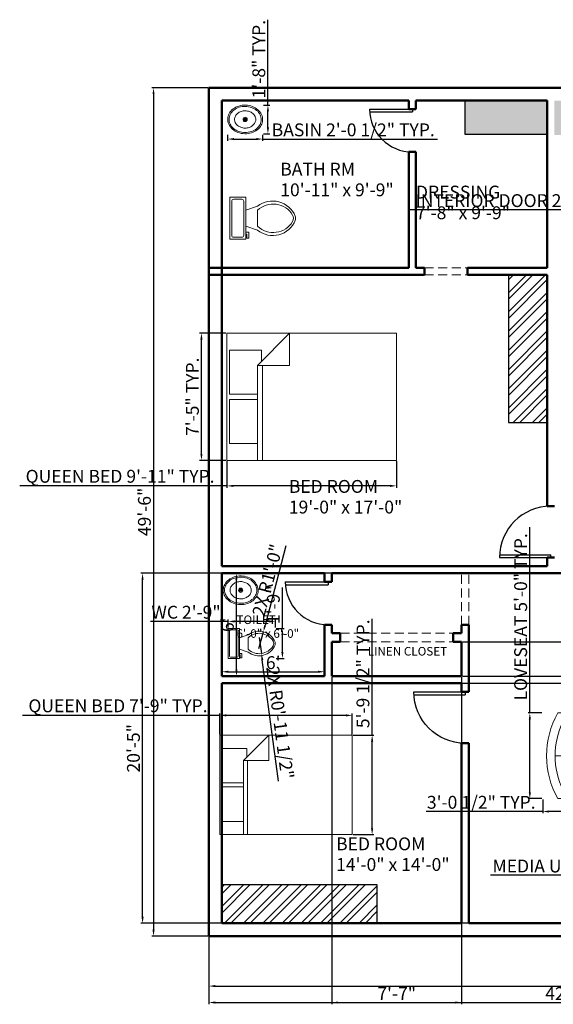
# Model space of a CAD drawing. Units: inches. Extents: x 2043 to 3102, y 1334 to 2053.
# Tile 1 of 4: x 2043 to 2416, y 1334 to 2024. Entities that reach past the tile are written whole.
import ezdxf

# ---------------------------------------------------------------- set-up
doc = ezdxf.new("R2010")
doc.units = ezdxf.units.IN
doc.linetypes.add('HIDDEN', pattern=[9.525, 6.35, -3.175])
for name, color, linetype, lineweight in [('A-ANNO-DIMS', 2, 'Continuous', 18), ('A-AREA-IDEN', 165, 'Continuous', 25), ('A-DOOR', 4, 'Continuous', 25), ('A-FLOR-CASE', 18, 'Continuous', 25), ('A-FLOR-CASE-PATT', 18, 'Continuous', 13), ('A-FLOR-FIXT', 9, 'Continuous', 20), ('A-FURN', 8, 'Continuous', 18), ('A-WALL', 7, 'Continuous', 50), ('A-WALL-OVHD', 11, 'HIDDEN', 18)]:
    doc.layers.add(name, color=color, linetype=linetype, lineweight=lineweight)
doc.styles.get("Standard").update_dxf_attribs({"font": 'arial.ttf'})
doc.dimstyles.new('ISO-25', dxfattribs={"dimtxt": 9, "dimasz": 4.5, "dimexe": 1.25, "dimexo": 0.625, "dimtad": 1, "dimdec": 0, "dimlunit": 3, "dimtxsty": 'Standard', "dimcen": 2.5, "dimadec": 0, "dimazin": 0, "dimtfac": 1, "dimtdec": 0, "dimtmove": 0, "dimatfit": 3, "dimfxl": 1, "dimarcsym": 0})

# ---------------------------------------------------------------- blocks, each defined once
blk = doc.blocks.new('Toilet - top')
for p, q in [((9.5, -6), (9.5, -2)), ((-10, -8.5), (-8, -8.5)), ((-10, -9.5), (-10, -8.5)), ((-7, -9.5), (-10, -9.5)), ((-8, -8.5), (-8, -8)), ((-7, -8), (-7, -9.5)), ((-4, -8), (-6, -14)), ((4, -8), (6, -14)), ((4, -14), (-4, -14))]:
    blk.add_line(p, q)
blk.add_lwpolyline([(10.5, -8), (10.5, 0), (-10.5, 0), (-10.5, -8)], close=True)
for points in [[(-9.5, -2), (-9.5, -6)], [(8.5, -1), (-8.5, -1)], [(-8.5, -7), (8.5, -7)]]:
    blk.add_lwpolyline(points)
for centre, radius, start, end in [((-8.62, -1.88), 0.884, 81.8699, 188.1301), ((8.62, -1.88), 0.884, 351.8699, 98.1301), ((-8.62, -6.12), 0.884, 171.8699, 278.1301), ((8.62, -6.12), 0.884, 261.8699, 8.1301), ((3.52, -21.58), 12.17, 141.4691, 247.9714), ((4.2, -21.82), 11.33, 136.3677, 238.9468), ((-3.52, -21.58), 12.17, 292.0284, 38.5307), ((-4.2, -21.82), 11.33, 301.053, 43.6321), ((0, -27.88), 4, 245.7318, 294.2682), ((0, -29), 4, 254.8605, 285.1395)]:
    blk.add_arc(centre, radius, start, end)
blk = doc.blocks.new('Bed - Queen')
for p, q in [((0, -80.00003), (0, 0)), ((0, 0), (59.99999, 0)), ((59.99999, 0), (59.99999, -80.00003)), ((7.99999, -1.2), (28.79998, -1.2)), ((7.99999, -14.4), (7.99999, -1.2)), ((28.79998, -1.2), (28.79998, -14.4)), ((31.19999, -1.2), (51.99999, -1.2)), ((31.19999, -14.4), (31.19999, -1.2)), ((51.99999, -1.2), (51.99999, -16.4)), ((0, -14.4), (44.8, -14.4)), ((44.8, -16.8), (0, -16.8)), ((59.99999, -29.6), (44.8, -14.4)), ((44.8, -14.4), (44.8, -29.6)), ((51.99999, -16.4), (46.79936, -16.4)), ((44.8, -29.6), (59.99999, -29.6)), ((59.99999, -80.00003), (0, -80.00003))]:
    blk.add_line(p, q)
blk = doc.blocks.new('Sofa - Roundback Loveseat 5 ft.')
for p, q in [((0, -32.44198), (0, -5.99998)), ((-24, -33.99998), (-24, -11.46958)), ((-23.9998, -13.38178), (23.99986, -13.38178)), ((24.00004, -33.99998), (24.00004, -11.46958)), ((-24, -32.44198), (24.00004, -32.44198))]:
    blk.add_line(p, q)
for points in [[(-24, -33.99998), (-30, -33.99998), (-30, -7.99998)], [(30.00004, -7.99998), (30.00004, -33.99998), (24.00004, -33.99998)]]:
    blk.add_lwpolyline(points)
for centre, radius, start, end in [((0, -60.24998), 60.24998, 60.13715, 119.8628), ((0, -61.38438), 55.38444, 64.32083, 115.6792)]:
    blk.add_arc(centre, radius, start, end)
blk = doc.blocks.new('Sink - Oval top')
for p, q in [((-1, 0), (1, 0)), ((0, 1), (0, -1))]:
    blk.add_line(p, q)
for points in [[(-12.23, 0.39, 0.117634), (-11.46, -3.36, 0.104469), (-8.88, -6.8, 0.090016), (-5.08, -9.07, 0.08192), (-0.32, -10.02, 0.08192), (4.49, -9.38, 0.090016), (8.42, -7.36, 0.104469), (11.22, -4.09, 0.117634), (12.23, -0.39, 0.117634), (11.46, 3.36, 0.104469), (8.88, 6.8, 0.090016), (5.08, 9.07, 0.08192), (0.32, 10.02, 0.08192), (-4.49, 9.38, 0.090016), (-8.42, 7.36, 0.104469), (-11.22, 4.09, 0.117634)], [(-11.29, 0.16, 0.118622), (-10.52, -3.25, 0.104678), (-8.07, -6.36, 0.089562), (-4.54, -8.37, 0.081185), (-0.13, -9.15, 0.081185), (4.3, -8.49, 0.089562), (7.89, -6.58, 0.104678), (10.42, -3.55, 0.118622), (11.29, -0.16, 0.118622), (10.52, 3.25, 0.104678), (8.07, 6.36, 0.089562), (4.54, 8.37, 0.081185), (0.13, 9.15, 0.081185), (-4.3, 8.49, 0.089562), (-7.89, 6.58, 0.104678), (-10.42, 3.55, 0.118622)], [(-7.42, 0.08, 0.118283), (-6.91, -2.17, 0.104607), (-5.29, -4.21, 0.089718), (-2.97, -5.53, 0.081436), (-0.07, -6.04, 0.081436), (2.84, -5.59, 0.089718), (5.2, -4.33, 0.104607), (6.86, -2.32, 0.118283), (7.42, -0.08, 0.118283), (6.91, 2.17, 0.104607), (5.29, 4.21, 0.089718), (2.97, 5.53, 0.081436), (0.07, 6.04, 0.081436), (-2.84, 5.59, 0.089718), (-5.2, 4.33, 0.104607), (-6.86, 2.32, 0.118283)]]:
    blk.add_lwpolyline(points, format="xyb", close=True)
for radius in [1.5, 1]:
    blk.add_circle((0, 0), radius)
blk = doc.blocks.new('*D17')
at = {"layer": 'A-ANNO-DIMS', "color": 0, "lineweight": -2, "transparency": 16777216}
for p, q in [((2222.37, 1636.25), (2193.2, 1636.25)), ((2194.45, 1568.75), (2194.45, 1631.75)), ((2219.56, 1564.25), (2193.2, 1564.25))]:
    blk.add_line(p, q, dxfattribs=at)
at = {"layer": 'A-ANNO-DIMS', "color": 0, "transparency": 16777216}
for points in [[(2193.7, 1631.75), (2195.2, 1631.75), (2194.45, 1636.25)], [(2193.7, 1568.75), (2195.2, 1568.75), (2194.45, 1564.25)]]:
    blk.add_solid(points, dxfattribs=at)
at = {"layer": 'Defpoints', "color": 0, "transparency": 16777216}
for p in [(2194.45, 1636.25), (2223, 1636.25), (2220.19, 1564.25)]:
    blk.add_point(p, dxfattribs=at)
at = {"layer": 'A-ANNO-DIMS', "color": 0, "transparency": 16777216, "insert": (2189.23, 1600.25), "char_height": 9, "attachment_point": 5, "rotation": 90}
blk.add_mtext("6'", dxfattribs=at)
blk = doc.blocks.new('*D18')
at = {"layer": 'A-ANNO-DIMS', "color": 0, "lineweight": -2, "transparency": 16777216}
for p, q in [((2184.19, 1570.54), (2184.19, 1566.09)), ((2188.69, 1567.34), (2251.69, 1567.34)), ((2256.19, 1568.32), (2256.19, 1566.09))]:
    blk.add_line(p, q, dxfattribs=at)
at = {"layer": 'A-ANNO-DIMS', "color": 0, "transparency": 16777216}
for points in [[(2188.69, 1568.09), (2188.69, 1566.59), (2184.19, 1567.34)], [(2251.69, 1568.09), (2251.69, 1566.59), (2256.19, 1567.34)]]:
    blk.add_solid(points, dxfattribs=at)
at = {"layer": 'Defpoints', "color": 0, "transparency": 16777216}
for p in [(2184.19, 1571.17), (2256.19, 1568.95), (2256.19, 1567.34)]:
    blk.add_point(p, dxfattribs=at)
at = {"layer": 'A-ANNO-DIMS', "color": 0, "transparency": 16777216, "insert": (2220.19, 1572.56), "char_height": 9, "attachment_point": 5}
blk.add_mtext("6'", dxfattribs=at)
blk = doc.blocks.new('*D19')
at = {"layer": 'A-ANNO-DIMS', "color": 0, "lineweight": -2, "transparency": 16777216}
for p, q in [((2174.56, 1976.25), (2135.12, 1976.25)), ((2136.37, 1971.75), (2136.37, 1386.75)), ((2174.56, 1382.25), (2135.12, 1382.25))]:
    blk.add_line(p, q, dxfattribs=at)
at = {"layer": 'A-ANNO-DIMS', "color": 0, "transparency": 16777216}
for points in [[(2135.62, 1971.75), (2137.12, 1971.75), (2136.37, 1976.25)], [(2135.62, 1386.75), (2137.12, 1386.75), (2136.37, 1382.25)]]:
    blk.add_solid(points, dxfattribs=at)
at = {"layer": 'Defpoints', "color": 0, "transparency": 16777216}
for p in [(2175.19, 1976.25), (2136.37, 1382.25), (2175.19, 1382.25)]:
    blk.add_point(p, dxfattribs=at)
at = {"layer": 'A-ANNO-DIMS', "color": 0, "transparency": 16777216, "insert": (2131.15, 1679.25), "char_height": 9, "attachment_point": 5, "rotation": 90}
blk.add_mtext('49\'-6"', dxfattribs=at)
blk = doc.blocks.new('*D20')
at = {"layer": 'A-ANNO-DIMS', "color": 0, "lineweight": -2, "transparency": 16777216}
for p, q in [((2175.19, 1381.63), (2175.19, 1346)), ((3054.19, 1381.63), (3054.19, 1346)), ((2179.69, 1347.25), (3049.69, 1347.25))]:
    blk.add_line(p, q, dxfattribs=at)
at = {"layer": 'A-ANNO-DIMS', "color": 0, "transparency": 16777216}
for points in [[(2179.69, 1348), (2179.69, 1346.5), (2175.19, 1347.25)], [(3049.69, 1348), (3049.69, 1346.5), (3054.19, 1347.25)]]:
    blk.add_solid(points, dxfattribs=at)
at = {"layer": 'Defpoints', "color": 0, "transparency": 16777216}
for p in [(2175.19, 1382.25), (3054.19, 1382.25), (3054.19, 1347.25)]:
    blk.add_point(p, dxfattribs=at)
at = {"layer": 'A-ANNO-DIMS', "color": 0, "transparency": 16777216, "insert": (2614.69, 1352.47), "char_height": 9, "attachment_point": 5}
blk.add_mtext('73\'-3"', dxfattribs=at)
blk = doc.blocks.new('DOOR-SWING-30IN')
for p, q in [((0, 30), (30, 30)), ((0, 28), (30, 28)), ((30, 30), (30, 28))]:
    blk.add_line(p, q)
blk.add_arc((30, 30), 30, 180, 270)
blk = doc.blocks.new('DOOR-SWING-36IN')
for p, q in [((0, 36), (0, 0)), ((2, 36), (2, 0)), ((0, 0), (2, 0))]:
    blk.add_line(p, q)
blk.add_arc((0, 0), 36, 0, 90)
blk = doc.blocks.new('*D24')
at = {"layer": 'A-ANNO-DIMS', "color": 0, "lineweight": -2, "transparency": 16777216}
for p, q in [((2187.75, 1714.67), (2187.75, 1696.22)), ((2306.57, 1714.67), (2306.57, 1696.22)), ((2187.75, 1697.47), (2042.62, 1697.47)), ((2302.07, 1697.47), (2192.25, 1697.47))]:
    blk.add_line(p, q, dxfattribs=at)
at = {"layer": 'A-ANNO-DIMS', "color": 0, "transparency": 16777216}
for points in [[(2192.25, 1698.22), (2192.25, 1696.72), (2187.75, 1697.47)], [(2302.07, 1698.22), (2302.07, 1696.72), (2306.57, 1697.47)]]:
    blk.add_solid(points, dxfattribs=at)
at = {"layer": 'Defpoints', "color": 0, "transparency": 16777216}
for p in [(2187.75, 1715.29), (2306.57, 1715.29), (2187.75, 1697.47)]:
    blk.add_point(p, dxfattribs=at)
at = {"layer": 'A-ANNO-DIMS', "color": 0, "transparency": 16777216, "insert": (2112.93, 1703.03), "char_height": 9, "attachment_point": 5}
blk.add_mtext('QUEEN BED 9\'-11" TYP.', dxfattribs=at)
blk = doc.blocks.new('*D25')
at = {"layer": 'A-ANNO-DIMS', "color": 0, "lineweight": -2, "transparency": 16777216}
for p, q in [((2187.13, 1804.41), (2168.68, 1804.41)), ((2169.93, 1719.79), (2169.93, 1799.91)), ((2187.13, 1715.29), (2168.68, 1715.29))]:
    blk.add_line(p, q, dxfattribs=at)
at = {"layer": 'A-ANNO-DIMS', "color": 0, "transparency": 16777216}
for points in [[(2169.18, 1799.91), (2170.68, 1799.91), (2169.93, 1804.41)], [(2169.18, 1719.79), (2170.68, 1719.79), (2169.93, 1715.29)]]:
    blk.add_solid(points, dxfattribs=at)
at = {"layer": 'Defpoints', "color": 0, "transparency": 16777216}
for p in [(2169.93, 1804.41), (2187.75, 1804.41), (2187.75, 1715.29)]:
    blk.add_point(p, dxfattribs=at)
at = {"layer": 'A-ANNO-DIMS', "color": 0, "transparency": 16777216, "insert": (2164.73, 1759.85), "char_height": 9, "attachment_point": 5, "rotation": 90}
blk.add_mtext('7\'-5" TYP.', dxfattribs=at)
blk = doc.blocks.new('*D26')
at = {"layer": 'A-ANNO-DIMS', "color": 0, "lineweight": -2, "transparency": 16777216}
for p, q in [((2182.79, 1523.5), (2182.79, 1538.04)), ((2275.57, 1523.5), (2275.57, 1538.04)), ((2182.79, 1536.79), (2044.65, 1536.79)), ((2271.07, 1536.79), (2187.29, 1536.79))]:
    blk.add_line(p, q, dxfattribs=at)
at = {"layer": 'A-ANNO-DIMS', "color": 0, "transparency": 16777216}
for points in [[(2187.29, 1537.54), (2187.29, 1536.04), (2182.79, 1536.79)], [(2271.07, 1537.54), (2271.07, 1536.04), (2275.57, 1536.79)]]:
    blk.add_solid(points, dxfattribs=at)
at = {"layer": 'Defpoints', "color": 0, "transparency": 16777216}
for p in [(2182.79, 1536.79), (2182.79, 1522.87), (2275.57, 1522.87)]:
    blk.add_point(p, dxfattribs=at)
at = {"layer": 'A-ANNO-DIMS', "color": 0, "transparency": 16777216, "insert": (2111.47, 1542.34), "char_height": 9, "attachment_point": 5}
blk.add_mtext('QUEEN BED 7\'-9" TYP.', dxfattribs=at)
blk = doc.blocks.new('*D27')
at = {"layer": 'A-ANNO-DIMS', "color": 0, "lineweight": -2, "transparency": 16777216}
for p, q in [((2289.49, 1522.87), (2289.49, 1604.45)), ((2276.2, 1522.87), (2290.74, 1522.87)), ((2289.49, 1457.79), (2289.49, 1518.37)), ((2276.2, 1453.29), (2290.74, 1453.29))]:
    blk.add_line(p, q, dxfattribs=at)
at = {"layer": 'A-ANNO-DIMS', "color": 0, "transparency": 16777216}
for points in [[(2288.74, 1518.37), (2290.24, 1518.37), (2289.49, 1522.87)], [(2288.74, 1457.79), (2290.24, 1457.79), (2289.49, 1453.29)]]:
    blk.add_solid(points, dxfattribs=at)
at = {"layer": 'Defpoints', "color": 0, "transparency": 16777216}
for p in [(2275.57, 1522.87), (2289.49, 1522.87), (2275.57, 1453.29)]:
    blk.add_point(p, dxfattribs=at)
at = {"layer": 'A-ANNO-DIMS', "color": 0, "transparency": 16777216, "insert": (2284.21, 1565.91), "char_height": 9, "attachment_point": 5, "rotation": 90}
blk.add_mtext('5\'-9 1/2" TYP.', dxfattribs=at)
blk = doc.blocks.new('*D28')
at = {"layer": 'A-ANNO-DIMS', "color": 0, "lineweight": -2, "transparency": 16777216}
for p, q in [((2188.26, 1943.35), (2188.26, 1939.04)), ((2192.76, 1940.29), (2208.31, 1940.29)), ((2212.81, 1943.35), (2212.81, 1939.04)), ((2212.81, 1940.29), (2335.22, 1940.29))]:
    blk.add_line(p, q, dxfattribs=at)
at = {"layer": 'A-ANNO-DIMS', "color": 0, "transparency": 16777216}
for points in [[(2192.76, 1941.04), (2192.76, 1939.54), (2188.26, 1940.29)], [(2208.31, 1941.04), (2208.31, 1939.54), (2212.81, 1940.29)]]:
    blk.add_solid(points, dxfattribs=at)
at = {"layer": 'Defpoints', "color": 0, "transparency": 16777216}
for p in [(2188.26, 1943.98), (2212.81, 1943.98), (2212.81, 1940.29)]:
    blk.add_point(p, dxfattribs=at)
at = {"layer": 'A-ANNO-DIMS', "color": 0, "transparency": 16777216, "insert": (2276.26, 1945.57), "char_height": 9, "attachment_point": 5}
blk.add_mtext('BASIN 2\'-0 1/2" TYP.', dxfattribs=at)
blk = doc.blocks.new('*D29')
at = {"layer": 'A-ANNO-DIMS', "color": 0, "lineweight": -2, "transparency": 16777216}
for p, q in [((2216.49, 1964.11), (2216.49, 2023.87)), ((2213.44, 1964.11), (2217.74, 1964.11)), ((2216.49, 1948.48), (2216.49, 1959.61)), ((2213.44, 1943.98), (2217.74, 1943.98))]:
    blk.add_line(p, q, dxfattribs=at)
at = {"layer": 'A-ANNO-DIMS', "color": 0, "transparency": 16777216}
for points in [[(2215.74, 1959.61), (2217.24, 1959.61), (2216.49, 1964.11)], [(2215.74, 1948.48), (2217.24, 1948.48), (2216.49, 1943.98)]]:
    blk.add_solid(points, dxfattribs=at)
at = {"layer": 'Defpoints', "color": 0, "transparency": 16777216}
for p in [(2212.81, 1964.11), (2216.49, 1964.11), (2212.81, 1943.98)]:
    blk.add_point(p, dxfattribs=at)
at = {"layer": 'A-ANNO-DIMS', "color": 0, "transparency": 16777216, "insert": (2211.27, 1996.24), "char_height": 9, "attachment_point": 5, "rotation": 90}
blk.add_mtext('1\'-8" TYP.', dxfattribs=at)
blk = doc.blocks.new('*D30')
at = {"layer": 'A-ANNO-DIMS', "color": 0, "lineweight": -2, "transparency": 16777216}
for p, q in [((2188.65, 1602.56), (2134.17, 1602.56)), ((2188.65, 1598.23), (2188.65, 1603.81)), ((2217.19, 1602.56), (2193.15, 1602.56)), ((2221.69, 1598.23), (2221.69, 1603.81))]:
    blk.add_line(p, q, dxfattribs=at)
at = {"layer": 'A-ANNO-DIMS', "color": 0, "transparency": 16777216}
for points in [[(2193.15, 1603.31), (2193.15, 1601.81), (2188.65, 1602.56)], [(2217.19, 1603.31), (2217.19, 1601.81), (2221.69, 1602.56)]]:
    blk.add_solid(points, dxfattribs=at)
at = {"layer": 'Defpoints', "color": 0, "transparency": 16777216}
for p in [(2188.65, 1602.56), (2188.65, 1597.61), (2221.69, 1597.61)]:
    blk.add_point(p, dxfattribs=at)
at = {"layer": 'A-ANNO-DIMS', "color": 0, "transparency": 16777216, "insert": (2159.16, 1607.84), "char_height": 9, "attachment_point": 5}
blk.add_mtext('WC 2\'-9"', dxfattribs=at)
blk = doc.blocks.new('*D31')
at = {"layer": 'A-ANNO-DIMS', "color": 0, "lineweight": -2, "transparency": 16777216}
for p, q in [((2226.65, 1597.61), (2226.65, 1626.43)), ((2222.32, 1597.61), (2227.9, 1597.61)), ((2226.65, 1581.11), (2226.65, 1593.11)), ((2222.32, 1576.61), (2227.9, 1576.61))]:
    blk.add_line(p, q, dxfattribs=at)
at = {"layer": 'A-ANNO-DIMS', "color": 0, "transparency": 16777216}
for points in [[(2225.9, 1593.11), (2227.4, 1593.11), (2226.65, 1597.61)], [(2225.9, 1581.11), (2227.4, 1581.11), (2226.65, 1576.61)]]:
    blk.add_solid(points, dxfattribs=at)
at = {"layer": 'Defpoints', "color": 0, "transparency": 16777216}
for p in [(2221.69, 1597.61), (2226.65, 1597.61), (2221.69, 1576.61)]:
    blk.add_point(p, dxfattribs=at)
at = {"layer": 'A-ANNO-DIMS', "color": 0, "transparency": 16777216, "insert": (2221.43, 1614.27), "char_height": 9, "attachment_point": 5, "rotation": 90}
blk.add_mtext('1\'-9"', dxfattribs=at)
blk = doc.blocks.new('*D34')
at = {"layer": 'A-ANNO-DIMS', "color": 0, "lineweight": -2, "transparency": 16777216}
for p, q in [((2479.69, 1890.75), (2314.95, 1890.75)), ((2479.69, 1886.88), (2479.69, 1892)), ((2505.19, 1890.75), (2484.19, 1890.75)), ((2509.69, 1886.88), (2509.69, 1892))]:
    blk.add_line(p, q, dxfattribs=at)
at = {"layer": 'A-ANNO-DIMS', "color": 0, "transparency": 16777216}
for points in [[(2484.19, 1891.5), (2484.19, 1890), (2479.69, 1890.75)], [(2505.19, 1891.5), (2505.19, 1890), (2509.69, 1890.75)]]:
    blk.add_solid(points, dxfattribs=at)
at = {"layer": 'Defpoints', "color": 0, "transparency": 16777216}
for p in [(2479.69, 1890.75), (2479.69, 1886.25), (2509.69, 1886.25)]:
    blk.add_point(p, dxfattribs=at)
at = {"layer": 'A-ANNO-DIMS', "color": 0, "transparency": 16777216, "insert": (2395.07, 1896.04), "char_height": 9, "attachment_point": 5}
blk.add_mtext('INTERIOR DOOR 2\'-6" TYP.', dxfattribs=at)
blk = doc.blocks.new('*D40')
at = {"layer": 'A-ANNO-DIMS', "color": 0, "lineweight": -2, "transparency": 16777216}
for p, q in [((2399.96, 1538.48), (2399.96, 1668.56)), ((2408.33, 1538.48), (2398.71, 1538.48)), ((2399.96, 1482.98), (2399.96, 1533.98)), ((2408.33, 1478.48), (2398.71, 1478.48))]:
    blk.add_line(p, q, dxfattribs=at)
at = {"layer": 'A-ANNO-DIMS', "color": 0, "transparency": 16777216}
for points in [[(2399.21, 1533.98), (2400.71, 1533.98), (2399.96, 1538.48)], [(2399.21, 1482.98), (2400.71, 1482.98), (2399.96, 1478.48)]]:
    blk.add_solid(points, dxfattribs=at)
at = {"layer": 'Defpoints', "color": 0, "transparency": 16777216}
for p in [(2399.96, 1538.48), (2408.96, 1538.48), (2408.96, 1478.48)]:
    blk.add_point(p, dxfattribs=at)
at = {"layer": 'A-ANNO-DIMS', "color": 0, "transparency": 16777216, "insert": (2394.68, 1605.77), "char_height": 9, "attachment_point": 5, "rotation": 90}
blk.add_mtext('LOVESEAT 5\'-0" TYP.', dxfattribs=at)
blk = doc.blocks.new('*D41')
at = {"layer": 'A-ANNO-DIMS', "color": 0, "lineweight": -2, "transparency": 16777216}
for p, q in [((2408.96, 1477.85), (2408.96, 1468.23)), ((2445.63, 1477.85), (2445.63, 1468.23)), ((2408.96, 1469.48), (2327.39, 1469.48)), ((2441.13, 1469.48), (2413.46, 1469.48))]:
    blk.add_line(p, q, dxfattribs=at)
at = {"layer": 'A-ANNO-DIMS', "color": 0, "transparency": 16777216}
for points in [[(2413.46, 1470.23), (2413.46, 1468.73), (2408.96, 1469.48)], [(2441.13, 1470.23), (2441.13, 1468.73), (2445.63, 1469.48)]]:
    blk.add_solid(points, dxfattribs=at)
at = {"layer": 'Defpoints', "color": 0, "transparency": 16777216}
for p in [(2408.96, 1478.48), (2445.63, 1478.48), (2408.96, 1469.48)]:
    blk.add_point(p, dxfattribs=at)
at = {"layer": 'A-ANNO-DIMS', "color": 0, "transparency": 16777216, "insert": (2365.92, 1474.76), "char_height": 9, "attachment_point": 5}
blk.add_mtext('3\'-0 1/2" TYP.', dxfattribs=at)
blk = doc.blocks.new('*D48')
at = {"layer": 'A-ANNO-DIMS', "color": 0, "lineweight": -2, "transparency": 16777216}
for p, q in [((2477.76, 1424.93), (2372.36, 1424.93)), ((2477.76, 1416.56), (2477.76, 1426.18)), ((2533.26, 1424.93), (2482.26, 1424.93)), ((2537.76, 1416.56), (2537.76, 1426.18))]:
    blk.add_line(p, q, dxfattribs=at)
at = {"layer": 'A-ANNO-DIMS', "color": 0, "transparency": 16777216}
for points in [[(2482.26, 1425.68), (2482.26, 1424.18), (2477.76, 1424.93)], [(2533.26, 1425.68), (2533.26, 1424.18), (2537.76, 1424.93)]]:
    blk.add_solid(points, dxfattribs=at)
at = {"layer": 'Defpoints', "color": 0, "transparency": 16777216}
for p in [(2477.76, 1424.93), (2477.76, 1415.93), (2537.76, 1415.93)]:
    blk.add_point(p, dxfattribs=at)
at = {"layer": 'A-ANNO-DIMS', "color": 0, "transparency": 16777216, "insert": (2422.81, 1430.15), "char_height": 9, "attachment_point": 5}
blk.add_mtext('MEDIA UNIT 5\'-0"', dxfattribs=at)
blk = doc.blocks.new('*D61')
at = {"layer": 'A-ANNO-DIMS', "color": 0, "lineweight": -2, "transparency": 16777216}
for p, q in [((2261.186555, 1563.629633), (2261.186555, 1334.494633)), ((2352.186555, 1563.629633), (2352.186555, 1334.494633)), ((2265.686555, 1335.744633), (2347.686555, 1335.744633))]:
    blk.add_line(p, q, dxfattribs=at)
at = {"layer": 'A-ANNO-DIMS', "color": 0, "transparency": 16777216}
for points in [[(2265.686555, 1336.494633), (2265.686555, 1334.994633), (2261.186555, 1335.744633)], [(2347.686555, 1336.494633), (2347.686555, 1334.994633), (2352.186555, 1335.744633)]]:
    blk.add_solid(points, dxfattribs=at)
at = {"layer": 'Defpoints', "color": 0, "transparency": 16777216}
for p in [(2261.186555, 1564.254633), (2352.186555, 1564.254633), (2352.186555, 1335.744633)]:
    blk.add_point(p, dxfattribs=at)
at = {"layer": 'A-ANNO-DIMS', "color": 0, "transparency": 16777216, "insert": (2306.686555, 1340.869633), "char_height": 9, "attachment_point": 5}
blk.add_mtext('7\'-7"', dxfattribs=at)
blk = doc.blocks.new('*D62')
at = {"layer": 'A-ANNO-DIMS', "color": 0, "lineweight": -2, "transparency": 16777216}
for p, q in [((3100.7, 1588.25), (3100.7, 1618.08)), ((2352.81, 1588.25), (3101.95, 1588.25)), ((3100.7, 1568.75), (3100.7, 1583.75)), ((2352.81, 1564.25), (3101.95, 1564.25))]:
    blk.add_line(p, q, dxfattribs=at)
at = {"layer": 'A-ANNO-DIMS', "color": 0, "transparency": 16777216}
for points in [[(3099.95, 1583.75), (3101.45, 1583.75), (3100.7, 1588.25)], [(3099.95, 1568.75), (3101.45, 1568.75), (3100.7, 1564.25)]]:
    blk.add_solid(points, dxfattribs=at)
at = {"layer": 'Defpoints', "color": 0, "transparency": 16777216}
for p in [(2352.19, 1588.25), (3100.7, 1588.25), (2352.19, 1564.25)]:
    blk.add_point(p, dxfattribs=at)
at = {"layer": 'A-ANNO-DIMS', "color": 0, "transparency": 16777216, "insert": (3095.48, 1605.42), "char_height": 9, "attachment_point": 5, "rotation": 90}
blk.add_mtext('2\'-0"', dxfattribs=at)
blk = doc.blocks.new('*D64')
at = {"layer": 'A-ANNO-DIMS', "color": 0, "lineweight": -2, "transparency": 16777216}
for p, q in [((3100.7, 1568.75), (3100.7, 1573.25)), ((2352.81, 1564.25), (3101.95, 1564.25)), ((2352.81, 1559.25), (3101.95, 1559.25)), ((3100.7, 1564.25), (3100.7, 1559.25)), ((3100.7, 1554.75), (3100.7, 1525.08))]:
    blk.add_line(p, q, dxfattribs=at)
at = {"layer": 'A-ANNO-DIMS', "color": 0, "transparency": 16777216}
for points in [[(3099.95, 1568.75), (3101.45, 1568.75), (3100.7, 1564.25)], [(3099.95, 1554.75), (3101.45, 1554.75), (3100.7, 1559.25)]]:
    blk.add_solid(points, dxfattribs=at)
at = {"layer": 'Defpoints', "color": 0, "transparency": 16777216}
for p in [(2352.19, 1564.25), (2352.19, 1559.25), (3100.7, 1559.25)]:
    blk.add_point(p, dxfattribs=at)
at = {"layer": 'A-ANNO-DIMS', "color": 0, "transparency": 16777216, "insert": (3095.48, 1537.67), "char_height": 9, "attachment_point": 5, "rotation": 90}
blk.add_mtext('0\'-5"', dxfattribs=at)
blk = doc.blocks.new('*D66')
at = {"layer": 'A-ANNO-DIMS', "color": 0, "lineweight": -2, "transparency": 16777216}
for p, q in [((2664.56, 1636.25), (2127.43, 1636.25)), ((2128.68, 1395.75), (2128.68, 1631.75)), ((2679.56, 1391.25), (2127.43, 1391.25))]:
    blk.add_line(p, q, dxfattribs=at)
at = {"layer": 'A-ANNO-DIMS', "color": 0, "transparency": 16777216}
for points in [[(2127.93, 1631.75), (2129.43, 1631.75), (2128.68, 1636.25)], [(2127.93, 1395.75), (2129.43, 1395.75), (2128.68, 1391.25)]]:
    blk.add_solid(points, dxfattribs=at)
at = {"layer": 'Defpoints', "color": 0, "transparency": 16777216}
for p in [(2128.68, 1636.25), (2665.19, 1636.25), (2680.19, 1391.25)]:
    blk.add_point(p, dxfattribs=at)
at = {"layer": 'A-ANNO-DIMS', "color": 0, "transparency": 16777216, "insert": (2123.46, 1513.75), "char_height": 9, "attachment_point": 5, "rotation": 90}
blk.add_mtext('20\'-5"', dxfattribs=at)
blk = doc.blocks.new('*D68')
at = {"layer": 'A-ANNO-DIMS', "color": 0, "lineweight": -2, "transparency": 16777216}
for p, q in [((2175.19, 1381.63), (2175.19, 1334.49)), ((2680.19, 1381.63), (2680.19, 1334.49)), ((2179.69, 1335.74), (2675.69, 1335.74))]:
    blk.add_line(p, q, dxfattribs=at)
at = {"layer": 'A-ANNO-DIMS', "color": 0, "transparency": 16777216}
for points in [[(2179.69, 1336.49), (2179.69, 1334.99), (2175.19, 1335.74)], [(2675.69, 1336.49), (2675.69, 1334.99), (2680.19, 1335.74)]]:
    blk.add_solid(points, dxfattribs=at)
at = {"layer": 'Defpoints', "color": 0, "transparency": 16777216}
for p in [(2175.19, 1382.25), (2680.19, 1382.25), (2680.19, 1335.74)]:
    blk.add_point(p, dxfattribs=at)
at = {"layer": 'A-ANNO-DIMS', "color": 0, "transparency": 16777216, "insert": (2427.69, 1340.89), "char_height": 9, "attachment_point": 5}
blk.add_mtext('42\'-1"', dxfattribs=at)
blk = doc.blocks.new('*D75')
at = {"layer": 'A-ANNO-DIMS', "color": 0, "lineweight": -2, "transparency": 16777216}
for p, q in [((2229.14, 1655.59), (2214.46, 1599.71)), ((2210.23, 1583.59), (2213.32, 1595.36))]:
    blk.add_line(p, q, dxfattribs=at)
at = {"layer": 'A-ANNO-DIMS', "color": 0, "transparency": 16777216}
blk.add_solid([(2213.74, 1599.9), (2215.19, 1599.52), (2213.32, 1595.36)], dxfattribs=at)
at = {"layer": 'Defpoints', "color": 0, "transparency": 16777216}
for p in [(2213.32, 1595.36), (2210.23, 1583.59)]:
    blk.add_point(p, dxfattribs=at)
at = {"layer": 'A-ANNO-DIMS', "color": 0, "transparency": 16777216, "insert": (2217.33, 1631.15), "char_height": 9, "attachment_point": 5, "rotation": 75.28199}
blk.add_mtext('2X R1\'-0"', dxfattribs=at)
blk = doc.blocks.new('*D76')
at = {"layer": 'A-ANNO-DIMS', "color": 0, "lineweight": -2, "transparency": 16777216}
for p, q in [((2210.47, 1591.31), (2211.97, 1580.08)), ((2224, 1490.64), (2212.57, 1575.62))]:
    blk.add_line(p, q, dxfattribs=at)
at = {"layer": 'A-ANNO-DIMS', "color": 0, "transparency": 16777216}
blk.add_solid([(2213.32, 1575.72), (2211.83, 1575.52), (2211.97, 1580.08)], dxfattribs=at)
at = {"layer": 'Defpoints', "color": 0, "transparency": 16777216}
for p in [(2210.47, 1591.31), (2211.97, 1580.08)]:
    blk.add_point(p, dxfattribs=at)
at = {"layer": 'A-ANNO-DIMS', "color": 0, "transparency": 16777216, "insert": (2223.82, 1531.6), "char_height": 9, "attachment_point": 5, "rotation": 277.65803}
blk.add_mtext('2X R0\'-11 1/2"', dxfattribs=at)

msp = doc.modelspace()

# ---------------------------------------------------------------- hatches: boundary and pattern name
at = {"layer": 'A-FLOR-CASE-PATT'}
h = msp.add_hatch(dxfattribs=at)
h.set_pattern_fill('ANSI36', color=256)
h.paths.add_polyline_path([(2412.19, 1967.25), (2354.72, 1967.25), (2354.72, 1943.39), (2412.19, 1943.39)])
h.paths.add_polyline_path([(2477.19, 1967.25), (2417.19, 1967.25), (2417.19, 1943.04), (2477.19, 1943.04)])
h.paths.add_polyline_path([(2812.19, 1967.25), (2752.19, 1967.25), (2752.19, 1943.42), (2812.19, 1943.42)])
h.paths.add_polyline_path([(2875.74, 1967.25), (2817.19, 1967.25), (2817.19, 1943.74), (2875.74, 1943.74)])
h = msp.add_hatch(dxfattribs=at)
h.set_pattern_fill('ANSI32', color=256)
h.paths.add_polyline_path([(2412.19, 1845.25), (2384.99, 1845.25), (2384.99, 1741.79), (2412.19, 1741.79)])
h.paths.add_polyline_path([(2845.19, 1845.25), (2817.19, 1845.25), (2817.19, 1753.98), (2845.19, 1753.98)])
h = msp.add_hatch(dxfattribs=at)
h.set_pattern_fill('ANSI32', color=256)
h.paths.add_polyline_path([(2293.13, 1418.11), (2184.19, 1418.11), (2184.19, 1391.25), (2293.13, 1391.25)])
h.paths.add_polyline_path([(2812.19, 1729.23), (2721.07, 1729.23), (2721.07, 1702.25), (2812.19, 1702.25)])
h.paths.add_polyline_path([(2612.19, 1729.38), (2508.87, 1729.38), (2508.87, 1702.25), (2612.19, 1702.25)])

# ---------------------------------------------------------------- linework, layer by layer
at = {"layer": 'A-FLOR-CASE'}
for p, q in [((2354.72, 1943.39), (2354.72, 1967.25)), ((2412.19, 1967.25), (2412.19, 1943.39)), ((2412.19, 1943.39), (2354.72, 1943.39)), ((2293.13, 1418.11), (2184.19, 1418.11)), ((2293.13, 1391.25), (2293.13, 1418.11)), ((2184.19, 1391.25), (2293.13, 1391.25))]:
    msp.add_line(p, q, dxfattribs=at)
msp.add_lwpolyline([(2384.99, 1845.25), (2384.99, 1741.79), (2412.19, 1741.79), (2412.19, 1845.25)], dxfattribs=at)
at = {"layer": 'A-WALL'}
for p, q in [((2175.19, 1976.25), (3054.19, 1976.25)), ((2175.19, 1976.25), (2175.19, 1382.25)), ((2184.19, 1967.25), (2315.19, 1967.25)), ((2184.19, 1967.25), (2184.19, 1641.25)), ((2315.19, 1967.25), (2315.19, 1961.25)), ((2320.19, 1967.25), (2320.19, 1961.25)), ((2320.19, 1967.25), (2412.19, 1967.25)), ((2412.19, 1967.25), (2412.19, 1850.25)), ((2315.19, 1961.25), (2320.19, 1961.25)), ((2315.19, 1931.25), (2315.19, 1850.25)), ((2315.19, 1931.25), (2320.19, 1931.25)), ((2320.19, 1931.25), (2320.19, 1850.25)), ((2175.19, 1850.25), (2315.19, 1850.25)), ((2320.19, 1850.25), (2326.19, 1850.25)), ((2326.19, 1850.25), (2326.19, 1845.25)), ((2356.19, 1850.25), (2412.19, 1850.25)), ((2356.19, 1850.25), (2356.19, 1845.25)), ((2175.19, 1845.25), (2326.19, 1845.25)), ((2356.19, 1845.25), (2412.19, 1845.25)), ((2412.19, 1845.25), (2412.19, 1683.25)), ((2412.19, 1683.25), (2417.19, 1683.25)), ((2184.19, 1641.25), (2412.19, 1641.25)), ((2412.19, 1647.25), (2417.19, 1647.25)), ((2412.19, 1647.25), (2412.19, 1641.25)), ((2184.19, 1636.25), (2256.19, 1636.25)), ((2184.19, 1636.25), (2184.19, 1564.25)), ((2256.19, 1636.25), (2256.19, 1630.25)), ((2261.19, 1636.25), (2261.19, 1630.25)), ((2261.19, 1636.25), (2665.19, 1636.25)), ((2256.19, 1630.25), (2261.19, 1630.25)), ((2256.19, 1600.25), (2261.19, 1600.25)), ((2256.19, 1600.25), (2256.19, 1564.25)), ((2261.19, 1600.25), (2261.19, 1594.25)), ((2352.19, 1600.25), (2357.19, 1600.25)), ((2352.19, 1594.25), (2352.19, 1600.25)), ((2357.19, 1559.25), (2357.19, 1600.25)), ((2261.19, 1594.25), (2267.19, 1594.25)), ((2267.19, 1594.25), (2267.19, 1588.25)), ((2346.19, 1594.25), (2352.19, 1594.25)), ((2346.19, 1588.25), (2346.19, 1594.25)), ((2261.19, 1588.25), (2267.19, 1588.25)), ((2261.19, 1588.25), (2261.19, 1564.25)), ((2346.19, 1588.25), (2352.19, 1588.25)), ((2352.19, 1564.25), (2352.19, 1588.25)), ((2184.19, 1564.25), (2256.19, 1564.25)), ((2184.19, 1559.25), (2352.19, 1559.25)), ((2184.19, 1559.25), (2184.19, 1391.25)), ((2261.19, 1564.25), (2352.19, 1564.25)), ((2352.19, 1559.25), (2352.19, 1553.25)), ((2357.19, 1564.25), (2357.19, 1553.25)), ((2352.19, 1553.25), (2357.19, 1553.25)), ((2352.19, 1517.25), (2357.19, 1517.25)), ((2352.19, 1517.25), (2352.19, 1391.25)), ((2357.19, 1517.25), (2357.19, 1391.25)), ((2184.19, 1391.25), (2352.19, 1391.25)), ((2357.19, 1391.25), (2680.19, 1391.25)), ((2175.19, 1382.25), (2680.19, 1382.25))]:
    msp.add_line(p, q, dxfattribs=at)
at = {"layer": 'A-WALL-OVHD'}
for p, q in [((2326.19, 1850.25), (2356.19, 1850.25)), ((2326.19, 1845.25), (2356.19, 1845.25)), ((2352.19, 1600.25), (2352.19, 1636.25)), ((2357.19, 1600.25), (2357.19, 1636.25)), ((2267.19, 1594.25), (2346.19, 1594.25)), ((2267.19, 1588.25), (2346.19, 1588.25))]:
    msp.add_line(p, q, dxfattribs=at)

# ---------------------------------------------------------------- block references
at = {"layer": 'A-DOOR'}
for p in [(2287.69, 1931.26), (2228.69, 1600.25)]:
    msp.add_blockref('DOOR-SWING-30IN', p, dxfattribs=at)
at = {"layer": 'A-DOOR', "rotation": 89.99999999999987}
msp.add_blockref('DOOR-SWING-36IN', (2414.69, 1647.26), dxfattribs=at)
at = {"layer": 'A-DOOR', "extrusion": (0, 0, -1), "zscale": -1, "rotation": 270}
msp.add_blockref('DOOR-SWING-36IN', (-2354.69, 1553.25), dxfattribs=at)
at = {"layer": 'A-FLOR-FIXT'}
for p in [(2200.54, 1954.04), (2197.42, 1624.41)]:
    msp.add_blockref('Sink - Oval top', p, dxfattribs=at)
at = {"layer": 'A-FLOR-FIXT', "xscale": 1.398246622267437, "yscale": 1.398246622267437, "zscale": 1.398246622267437, "rotation": 90}
msp.add_blockref('Toilet - top', (2189.73, 1884.83), dxfattribs=at)
at = {"layer": 'A-FLOR-FIXT', "rotation": 90}
msp.add_blockref('Toilet - top', (2188.65, 1587.11), dxfattribs=at)
at = {"layer": 'A-FURN'}
for p, xscale, yscale, zscale, rotation in [((2187.75, 1715.29), 1.485242787327834, 1.485242787327834, 1.485242787327834, 89.99999999999999), ((2182.79, 1453.29), 1.159729474409778, 1.159729474409778, 1.159729474409778, 90)]:
    msp.add_blockref('Bed - Queen', p, dxfattribs=dict(at, xscale=xscale, yscale=yscale, zscale=zscale, rotation=rotation))
at = {"layer": 'A-FURN', "rotation": 90}
msp.add_blockref('Sofa - Roundback Loveseat 5 ft.', (2411.63, 1508.48), dxfattribs=at)

# ---------------------------------------------------------------- texts
at = {"layer": 'A-AREA-IDEN'}
for s, height, p in [('BATH RM', 9, (2225.14, 1914.71)), ('10\'-11" x 9\'-9"', 9, (2225.14, 1900.25)), ('DRESSING ', 9, (2320.19, 1898.66)), ('7\'-8" x 9\'-9"', 9, (2320.19, 1884.2)), ('BED ROOM ', 9, (2231.14, 1692.59)), ('19\'-0" x 17\'-0"', 9, (2231.14, 1678.13)), ('TOILET', 6, (2194.49, 1600.74)), ('6\'-0" x 6\'-0"', 6, (2194.49, 1591.1)), ('LINEN CLOSET', 6, (2286.38, 1578.67)), ('BED ROOM ', 9, (2264.27, 1442.33)), ('14\'-0" x 14\'-0"', 9, (2264.27, 1427.88))]:
    msp.add_text(s, height=height, dxfattribs=at).set_placement(p)

# ---------------------------------------------------------------- dimensions: what is measured, and where the dimension line sits
at = {"layer": 'A-ANNO-DIMS'}
for base, p1, p2, angle, text, picture, middle in [((2216.49, 1964.11), (2212.81, 1943.98), (2212.81, 1964.11), 90, '<> TYP.', '*D29', (2211.27, 1996.24)), ((2479.69, 1890.75), (2509.69, 1886.25), (2479.69, 1886.25), 180, 'INTERIOR DOOR <> TYP.', '*D34', (2395.07, 1896.04)), ((2169.93, 1804.41), (2187.75, 1715.29), (2187.75, 1804.41), 90, '<> TYP.', '*D25', (2164.73, 1759.85)), ((2187.75, 1697.47), (2306.57, 1715.29), (2187.75, 1715.29), 180, 'QUEEN BED <> TYP.', '*D24', (2112.93, 1703.03)), ((2399.96, 1538.48), (2408.96, 1478.48), (2408.96, 1538.48), 90, 'LOVESEAT <> TYP.', '*D40', (2394.68, 1605.77)), ((2188.65, 1602.56), (2221.69, 1597.61), (2188.65, 1597.61), 180, 'WC <>', '*D30', (2159.16, 1607.84)), ((2289.49, 1522.87), (2275.57, 1453.29), (2275.57, 1522.87), 90, '<> TYP.', '*D27', (2284.21, 1565.91)), ((2182.79, 1536.79), (2275.57, 1522.87), (2182.79, 1522.87), 180, 'QUEEN BED <> TYP.', '*D26', (2111.47, 1542.34)), ((2408.96, 1469.48), (2445.63, 1478.48), (2408.96, 1478.48), 180, '<> TYP.', '*D41', (2365.92, 1474.76)), ((2477.76, 1424.93), (2537.76, 1415.93), (2477.76, 1415.93), 180, 'MEDIA UNIT <>', '*D48', (2422.81, 1430.15))]:
    dim = msp.add_linear_dim(base=base, p1=p1, p2=p2, angle=angle, text=text, dimstyle='ISO-25', override={"dimdec": 1, "dimlfac": 1, "dimrnd": 0, "dimzin": 1, "dimdsep": 46, "dimlunit": 4, "dimfrac": 2}, dxfattribs=at)
    dim.commit()
    dim.dimension.update_dxf_attribs({"geometry": picture, "text_midpoint": middle})
for base, p1, p2, override, picture, middle in [((2136.37, 1382.25), (2175.19, 1976.25), (2175.19, 1382.25), {"dimclrd": 0, "dimclre": 0, "dimclrt": 0}, '*D19', (2131.15, 1679.25)), ((2128.68, 1636.25), (2680.19, 1391.25), (2665.19, 1636.25), {"dimdec": 1, "dimlfac": 1, "dimrnd": 0, "dimzin": 1, "dimdsep": 46, "dimlunit": 4, "dimfrac": 2}, '*D66', (2123.46, 1513.75)), ((2194.45, 1636.25), (2220.19, 1564.25), (2223, 1636.25), {"dimclrd": 0, "dimclre": 0, "dimclrt": 0}, '*D17', (2189.23, 1600.25)), ((2226.65, 1597.61), (2221.69, 1576.61), (2221.69, 1597.61), {"dimdec": 1, "dimlfac": 1, "dimrnd": 0, "dimzin": 1, "dimdsep": 46, "dimlunit": 4, "dimfrac": 2}, '*D31', (2221.43, 1614.27)), ((3100.7, 1588.25), (2352.19, 1564.25), (2352.19, 1588.25), {"dimdec": 1, "dimlfac": 1, "dimrnd": 0, "dimzin": 1, "dimdsep": 46, "dimlunit": 4, "dimfrac": 2}, '*D62', (3095.48, 1605.42)), ((3100.7, 1559.25), (2352.19, 1564.25), (2352.19, 1559.25), {"dimdec": 1, "dimlfac": 1, "dimrnd": 0, "dimzin": 1, "dimdsep": 46, "dimlunit": 4, "dimfrac": 2}, '*D64', (3095.48, 1537.67))]:
    dim = msp.add_linear_dim(base=base, p1=p1, p2=p2, angle=90, dimstyle='ISO-25', override=override, dxfattribs=at)
    dim.commit()
    dim.dimension.update_dxf_attribs({"geometry": picture, "text_midpoint": middle})
dim = msp.add_linear_dim(base=(2212.811, 1940.2934), p1=(2188.2601, 1943.9761), p2=(2212.811, 1943.9761), text='BASIN <> TYP.', dimstyle='ISO-25', override={"dimdec": 1, "dimlfac": 1, "dimrnd": 0, "dimzin": 1, "dimdsep": 46, "dimlunit": 4, "dimfrac": 2}, dxfattribs=at)
dim.commit()
dim.dimension.update_dxf_attribs({"geometry": '*D28', "text_midpoint": (2276.2641, 1945.5719)})
for center, mpoint, picture, middle in [((2210.23, 1583.59), (2213.32, 1595.36), '*D75', (2217.33, 1631.15)), ((2210.47, 1591.31), (2211.97, 1580.08), '*D76', (2223.82, 1531.6))]:
    dim = msp.add_radius_dim(center=center, mpoint=mpoint, text='2X <>', dimstyle='ISO-25', override={"dimdec": 1, "dimlfac": 1, "dimrnd": 0, "dimzin": 1, "dimdsep": 46, "dimlunit": 4, "dimfrac": 2}, dxfattribs=at)
    dim.commit()
    dim.dimension.update_dxf_attribs({"geometry": picture, "text_midpoint": middle})
for base, p1, p2, override, picture, middle in [((2256.19, 1567.34), (2184.19, 1571.17), (2256.19, 1568.95), {"dimclrd": 0, "dimclre": 0, "dimclrt": 0}, '*D18', (2220.19, 1572.56)), ((2352.19, 1335.74), (2261.19, 1564.25), (2352.19, 1564.25), {"dimdec": 1, "dimlfac": 1, "dimrnd": 0, "dimzin": 1, "dimdsep": 46, "dimlunit": 4, "dimfrac": 2}, '*D61', (2306.69, 1340.87)), ((3054.19, 1347.25), (2175.19, 1382.25), (3054.19, 1382.25), {"dimclrd": 0, "dimclre": 0, "dimclrt": 0}, '*D20', (2614.69, 1352.47)), ((2680.19, 1335.74), (2175.19, 1382.25), (2680.19, 1382.25), {"dimdec": 1, "dimlfac": 1, "dimrnd": 0, "dimzin": 1, "dimdsep": 46, "dimlunit": 4, "dimfrac": 2}, '*D68', (2427.69, 1340.89))]:
    dim = msp.add_linear_dim(base=base, p1=p1, p2=p2, dimstyle='ISO-25', override=override, dxfattribs=at)
    dim.commit()
    dim.dimension.update_dxf_attribs({"geometry": picture, "text_midpoint": middle})

doc.saveas('drawing.dxf')
